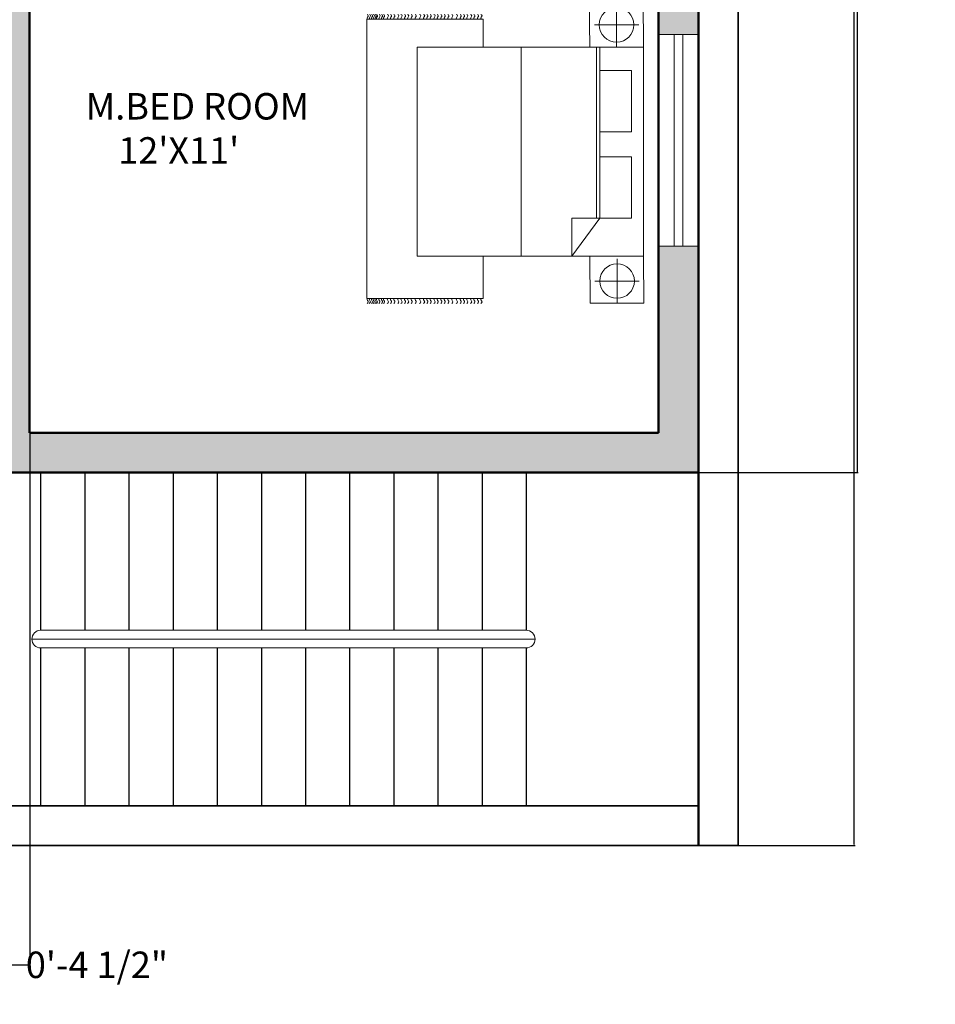
# Model space of a CAD drawing. Units: inches. Extents: x 3398 to 3816, y 15195 to 15771.
# Tile 6 of 10: x 3608 to 3816, y 15195 to 15418. Entities that reach past the tile are written whole.
import ezdxf

# ---------------------------------------------------------------- set-up
doc = ezdxf.new("R2010")
doc.units = ezdxf.units.IN
doc.header["$MEASUREMENT"] = 0
for name, color, linetype, lineweight in [('A-ANNO-DIMS', 2, 'Continuous', 18), ('A-AREA-IDEN', 7, 'Continuous', 25), ('A-FLOR-RAIL', 201, 'Continuous', 18), ('A-FLOR-STRS', 7, 'Continuous', 25), ('A-FURN', 8, 'Continuous', 18), ('A-GLAZ', 4, 'Continuous', 18), ('A-WALL', 7, 'Continuous', 50), ('A-WALL-PATT', 252, 'Continuous', 13), ('C-PROP', 7, 'Continuous', 35)]:
    doc.layers.add(name, color=color, linetype=linetype, lineweight=lineweight)
doc.styles.get("Standard").update_dxf_attribs({"font": 'arial.ttf'})
doc.dimstyles.get("Standard").update_dxf_attribs({"dimtxt": 6, "dimasz": 0.18, "dimexe": 0.18, "dimexo": 0.0625, "dimgap": 0.09, "dimtad": 0, "dimtih": 1, "dimtoh": 1, "dimdec": 1, "dimzin": 0, "dimdsep": 46, "dimlunit": 3, "dimtxsty": 'Standard', "dimcen": 0.09, "dimadec": 0, "dimazin": 0, "dimtfac": 1, "dimtdec": 1, "dimtofl": 0, "dimtmove": 0, "dimatfit": 3, "dimfxl": 1, "dimtolj": 1, "dimtzin": 0, "dimarcsym": 0})

# ---------------------------------------------------------------- blocks, each defined once
blk = doc.blocks.new('*D5')
at = {"layer": 'A-ANNO-DIMS', "color": 0, "lineweight": -2, "transparency": 16777216}
for p, q in [((3771.25, 15739.52), (3797.69, 15739.52)), ((3797.51, 15739.34), (3797.51, 15488.17)), ((3797.51, 15230.7), (3797.51, 15481.87)), ((3771.25, 15230.52), (3797.69, 15230.52))]:
    blk.add_line(p, q, dxfattribs=at)
at = {"layer": 'A-ANNO-DIMS', "color": 0, "transparency": 16777216}
for points in [[(3797.48, 15739.34), (3797.54, 15739.34), (3797.51, 15739.52)], [(3797.48, 15230.7), (3797.54, 15230.7), (3797.51, 15230.52)]]:
    blk.add_solid(points, dxfattribs=at)
at = {"layer": 'Defpoints', "color": 0, "transparency": 16777216}
for p in [(3771.19, 15739.52), (3771.19, 15230.52), (3797.51, 15230.52)]:
    blk.add_point(p, dxfattribs=at)
at = {"layer": 'A-ANNO-DIMS', "color": 0, "transparency": 16777216, "insert": (3797.51, 15485.02), "char_height": 6, "attachment_point": 5}
blk.add_mtext('\\A1;42\'-5.0"', dxfattribs=at)
blk = doc.blocks.new('BED-DOUBLE-WITH-NIGHTSTANDS')
for p, q in [((56.59, 58.08), (56.59, 68.14)), ((0, 64.36), (26.37, 64.36)), ((0, 1.12), (0, 64.36)), ((26.37, 64.36), (26.37, 58.06)), ((61.62, 63.11), (51.56, 63.11)), ((34.96, 10.66), (34.96, 58.08)), ((52, 19.27), (52, 58.08)), ((52.82, 19.32), (52.82, 58.08)), ((52.82, 19.32), (46.47, 10.71)), ((52.82, 19.27), (46.47, 19.27)), ((46.47, 19.27), (46.47, 10.71)), ((26.37, 10.66), (26.37, 1.12)), ((56.69, 0.03), (56.69, 10.09)), ((61.72, 5.06), (51.66, 5.06)), ((26.37, 1.12), (0, 1.12))]:
    blk.add_line(p, q)
for points in [[(50.39, 68.71), (50.5, 58.08), (62.68, 58.08), (62.58, 68.71)], [(62.68, 10.66), (11.37, 10.66), (11.37, 58.08), (62.68, 58.08)], [(59.98, 38.83), (52.82, 38.83), (52.82, 52.73), (59.98, 52.73)], [(59.98, 19.27), (52.82, 19.27), (52.82, 33.16), (59.98, 33.16)], [(50.5, 10.66), (50.6, 0.03), (62.78, 0.03), (62.68, 10.66)]]:
    blk.add_lwpolyline(points, close=True)
for centre in [(56.59, 63.11), (56.69, 5.06)]:
    blk.add_circle(centre, 3.92)
for points, knots in [([(0.07, 65.48), (0.19, 65.39), (0.43, 65.19), (0.19, 64.85), (0.02, 64.57), (0.13, 64.42), (0.18, 64.36)], [0, 0, 0, 0, 0.400747, 0.791423, 1.067667, 1.29709, 1.29709, 1.29709, 1.29709]), ([(0.57, 65.48), (0.7, 65.39), (0.94, 65.19), (0.7, 64.85), (0.52, 64.57), (0.63, 64.42), (0.68, 64.36)], [0, 0, 0, 0, 0.400747, 0.791423, 1.067667, 1.29709, 1.29709, 1.29709, 1.29709]), ([(1.06, 65.48), (1.18, 65.39), (1.42, 65.19), (1.18, 64.85), (1.01, 64.57), (1.11, 64.42), (1.16, 64.36)], [0, 0, 0, 0, 0.400747, 0.791423, 1.067667, 1.29709, 1.29709, 1.29709, 1.29709]), ([(1.46, 65.48), (1.58, 65.39), (1.82, 65.19), (1.58, 64.85), (1.41, 64.57), (1.51, 64.42), (1.56, 64.36)], [0, 0, 0, 0, 0.400747, 0.791423, 1.067667, 1.29709, 1.29709, 1.29709, 1.29709]), ([(1.88, 65.48), (2, 65.39), (2.24, 65.19), (2, 64.85), (1.82, 64.57), (1.93, 64.42), (1.98, 64.36)], [0, 0, 0, 0, 0.400747, 0.791423, 1.067667, 1.29709, 1.29709, 1.29709, 1.29709]), ([(2.18, 65.48), (2.31, 65.39), (2.55, 65.19), (2.31, 64.85), (2.13, 64.57), (2.24, 64.42), (2.29, 64.36)], [0, 0, 0, 0, 0.400747, 0.791423, 1.067667, 1.29709, 1.29709, 1.29709, 1.29709]), ([(2.76, 65.48), (2.88, 65.39), (3.12, 65.19), (2.88, 64.85), (2.71, 64.57), (2.81, 64.42), (2.86, 64.36)], [0, 0, 0, 0, 0.400747, 0.791423, 1.067667, 1.29709, 1.29709, 1.29709, 1.29709]), ([(3.33, 65.48), (3.45, 65.39), (3.7, 65.2), (3.44, 64.85), (3.27, 64.57), (3.38, 64.42), (3.43, 64.36)], [0, 0, 0, 0, 0.407265, 0.802015, 1.07826, 1.307683, 1.307683, 1.307683, 1.307683]), ([(3.75, 65.48), (3.88, 65.39), (4.12, 65.19), (3.88, 64.85), (3.7, 64.57), (3.81, 64.42), (3.86, 64.36)], [0, 0, 0, 0, 0.400747, 0.791423, 1.067667, 1.29709, 1.29709, 1.29709, 1.29709]), ([(4.64, 65.48), (4.76, 65.39), (5, 65.19), (4.76, 64.85), (4.59, 64.57), (4.69, 64.42), (4.74, 64.36)], [0, 0, 0, 0, 0.400747, 0.791423, 1.067667, 1.29709, 1.29709, 1.29709, 1.29709]), ([(5.36, 65.48), (5.49, 65.39), (5.73, 65.19), (5.49, 64.85), (5.31, 64.57), (5.42, 64.42), (5.47, 64.36)], [0, 0, 0, 0, 0.400747, 0.791423, 1.067667, 1.29709, 1.29709, 1.29709, 1.29709]), ([(6.12, 65.48), (6.24, 65.39), (6.48, 65.19), (6.24, 64.85), (6.07, 64.57), (6.17, 64.42), (6.22, 64.36)], [0, 0, 0, 0, 0.400747, 0.791423, 1.067667, 1.29709, 1.29709, 1.29709, 1.29709]), ([(7, 65.48), (7.12, 65.39), (7.36, 65.19), (7.12, 64.85), (6.95, 64.57), (7.05, 64.42), (7.1, 64.36)], [0, 0, 0, 0, 0.400747, 0.791423, 1.067667, 1.29709, 1.29709, 1.29709, 1.29709]), ([(7.73, 65.48), (7.85, 65.39), (8.09, 65.19), (7.85, 64.85), (7.68, 64.57), (7.78, 64.42), (7.83, 64.36)], [0, 0, 0, 0, 0.400747, 0.791423, 1.067667, 1.29709, 1.29709, 1.29709, 1.29709]), ([(8.54, 65.48), (8.66, 65.39), (8.9, 65.19), (8.66, 64.85), (8.49, 64.57), (8.6, 64.42), (8.65, 64.36)], [0, 0, 0, 0, 0.400747, 0.791423, 1.067667, 1.29709, 1.29709, 1.29709, 1.29709]), ([(9.23, 65.48), (9.35, 65.39), (9.59, 65.19), (9.35, 64.85), (9.18, 64.57), (9.29, 64.42), (9.34, 64.36)], [0, 0, 0, 0, 0.400747, 0.791423, 1.067667, 1.29709, 1.29709, 1.29709, 1.29709]), ([(10.05, 65.48), (10.17, 65.39), (10.41, 65.19), (10.17, 64.85), (10, 64.57), (10.1, 64.42), (10.15, 64.36)], [0, 0, 0, 0, 0.400747, 0.791423, 1.067667, 1.29709, 1.29709, 1.29709, 1.29709]), ([(10.93, 65.48), (11.05, 65.39), (11.29, 65.19), (11.05, 64.85), (10.88, 64.57), (10.99, 64.42), (11.03, 64.36)], [0, 0, 0, 0, 0.400747, 0.791423, 1.067667, 1.29709, 1.29709, 1.29709, 1.29709]), ([(11.97, 65.48), (12.09, 65.39), (12.33, 65.19), (12.09, 64.85), (11.92, 64.57), (12.02, 64.42), (12.07, 64.36)], [0, 0, 0, 0, 0.400747, 0.791423, 1.067667, 1.29709, 1.29709, 1.29709, 1.29709]), ([(12.85, 65.48), (12.97, 65.39), (13.21, 65.19), (12.97, 64.85), (12.8, 64.57), (12.9, 64.42), (12.95, 64.36)], [0, 0, 0, 0, 0.400747, 0.791423, 1.067667, 1.29709, 1.29709, 1.29709, 1.29709]), ([(13.58, 65.48), (13.7, 65.39), (13.94, 65.19), (13.7, 64.85), (13.53, 64.57), (13.63, 64.42), (13.68, 64.36)], [0, 0, 0, 0, 0.400747, 0.791423, 1.067667, 1.29709, 1.29709, 1.29709, 1.29709]), ([(14.33, 65.48), (14.45, 65.39), (14.69, 65.19), (14.45, 64.85), (14.28, 64.57), (14.38, 64.42), (14.43, 64.36)], [0, 0, 0, 0, 0.400747, 0.791423, 1.067667, 1.29709, 1.29709, 1.29709, 1.29709]), ([(15.21, 65.48), (15.33, 65.39), (15.57, 65.19), (15.33, 64.85), (15.16, 64.57), (15.27, 64.42), (15.32, 64.36)], [0, 0, 0, 0, 0.400747, 0.791423, 1.067667, 1.29709, 1.29709, 1.29709, 1.29709]), ([(15.94, 65.48), (16.06, 65.39), (16.3, 65.19), (16.06, 64.85), (15.89, 64.57), (16, 64.42), (16.04, 64.36)], [0, 0, 0, 0, 0.400747, 0.791423, 1.067667, 1.29709, 1.29709, 1.29709, 1.29709]), ([(16.76, 65.48), (16.88, 65.39), (17.12, 65.19), (16.88, 64.85), (16.7, 64.57), (16.81, 64.42), (16.86, 64.36)], [0, 0, 0, 0, 0.400747, 0.791423, 1.067667, 1.29709, 1.29709, 1.29709, 1.29709]), ([(17.53, 65.48), (17.65, 65.39), (17.89, 65.19), (17.65, 64.85), (17.48, 64.57), (17.59, 64.42), (17.64, 64.36)], [0, 0, 0, 0, 0.400747, 0.791423, 1.067667, 1.29709, 1.29709, 1.29709, 1.29709]), ([(18.35, 65.48), (18.47, 65.39), (18.71, 65.19), (18.47, 64.85), (18.3, 64.57), (18.4, 64.42), (18.45, 64.36)], [0, 0, 0, 0, 0.400747, 0.791423, 1.067667, 1.29709, 1.29709, 1.29709, 1.29709]), ([(19.23, 65.48), (19.35, 65.39), (19.59, 65.19), (19.35, 64.85), (19.18, 64.57), (19.29, 64.42), (19.33, 64.36)], [0, 0, 0, 0, 0.400747, 0.791423, 1.067667, 1.29709, 1.29709, 1.29709, 1.29709]), ([(20.27, 65.48), (20.39, 65.39), (20.63, 65.19), (20.39, 64.85), (20.22, 64.57), (20.32, 64.42), (20.37, 64.36)], [0, 0, 0, 0, 0.400747, 0.791423, 1.067667, 1.29709, 1.29709, 1.29709, 1.29709]), ([(21.15, 65.48), (21.27, 65.39), (21.51, 65.19), (21.27, 64.85), (21.1, 64.57), (21.21, 64.42), (21.25, 64.36)], [0, 0, 0, 0, 0.400747, 0.791423, 1.067667, 1.29709, 1.29709, 1.29709, 1.29709]), ([(21.88, 65.48), (22, 65.39), (22.24, 65.19), (22, 64.85), (21.83, 64.57), (21.93, 64.42), (21.98, 64.36)], [0, 0, 0, 0, 0.400747, 0.791423, 1.067667, 1.29709, 1.29709, 1.29709, 1.29709]), ([(22.63, 65.48), (22.75, 65.39), (22.99, 65.19), (22.75, 64.85), (22.58, 64.57), (22.69, 64.42), (22.73, 64.36)], [0, 0, 0, 0, 0.400747, 0.791423, 1.067667, 1.29709, 1.29709, 1.29709, 1.29709]), ([(23.51, 65.48), (23.63, 65.39), (23.87, 65.19), (23.63, 64.85), (23.46, 64.57), (23.57, 64.42), (23.62, 64.36)], [0, 0, 0, 0, 0.400747, 0.791423, 1.067667, 1.29709, 1.29709, 1.29709, 1.29709]), ([(24.24, 65.48), (24.36, 65.39), (24.6, 65.19), (24.36, 64.85), (24.19, 64.57), (24.3, 64.42), (24.34, 64.36)], [0, 0, 0, 0, 0.400747, 0.791423, 1.067667, 1.29709, 1.29709, 1.29709, 1.29709]), ([(25.06, 65.48), (25.18, 65.39), (25.42, 65.19), (25.18, 64.85), (25.01, 64.57), (25.11, 64.42), (25.16, 64.36)], [0, 0, 0, 0, 0.400747, 0.791423, 1.067667, 1.29709, 1.29709, 1.29709, 1.29709]), ([(25.84, 65.48), (25.96, 65.39), (26.2, 65.19), (25.96, 64.85), (25.78, 64.57), (25.89, 64.42), (25.94, 64.36)], [0, 0, 0, 0, 0.400747, 0.791423, 1.067667, 1.29709, 1.29709, 1.29709, 1.29709]), ([(0.07, 0), (0.19, 0.1), (0.43, 0.29), (0.19, 0.63), (0.02, 0.91), (0.13, 1.06), (0.18, 1.13)], [0, 0, 0, 0, 0.400747, 0.791423, 1.067667, 1.29709, 1.29709, 1.29709, 1.29709]), ([(0.55, 0), (0.67, 0.1), (0.91, 0.29), (0.67, 0.63), (0.49, 0.91), (0.6, 1.06), (0.65, 1.13)], [0, 0, 0, 0, 0.400747, 0.791423, 1.067667, 1.29709, 1.29709, 1.29709, 1.29709]), ([(1.03, 0), (1.15, 0.1), (1.39, 0.29), (1.15, 0.63), (0.98, 0.91), (1.09, 1.06), (1.13, 1.13)], [0, 0, 0, 0, 0.400747, 0.791423, 1.067667, 1.29709, 1.29709, 1.29709, 1.29709]), ([(1.43, 0), (1.55, 0.1), (1.79, 0.29), (1.55, 0.63), (1.38, 0.91), (1.48, 1.06), (1.53, 1.13)], [0, 0, 0, 0, 0.400747, 0.791423, 1.067667, 1.29709, 1.29709, 1.29709, 1.29709]), ([(1.85, 0), (1.97, 0.1), (2.21, 0.29), (1.97, 0.63), (1.8, 0.91), (1.9, 1.05), (1.94, 1.12)], [0, 0, 0, 0, 0.400747, 0.791423, 1.067667, 1.283686, 1.283686, 1.283686, 1.283686]), ([(2.16, 0), (2.28, 0.1), (2.52, 0.29), (2.28, 0.63), (2.11, 0.91), (2.21, 1.05), (2.25, 1.12)], [0, 0, 0, 0, 0.400747, 0.791423, 1.067667, 1.283686, 1.283686, 1.283686, 1.283686]), ([(2.73, 0), (2.85, 0.1), (3.09, 0.29), (2.85, 0.63), (2.68, 0.91), (2.78, 1.05), (2.82, 1.12)], [0, 0, 0, 0, 0.400747, 0.791423, 1.067667, 1.283686, 1.283686, 1.283686, 1.283686]), ([(3.33, 0), (3.45, 0.1), (3.69, 0.29), (3.45, 0.63), (3.27, 0.91), (3.38, 1.05), (3.42, 1.12)], [0, 0, 0, 0, 0.402903, 0.794912, 1.071156, 1.287177, 1.287177, 1.287177, 1.287177]), ([(3.75, 0), (3.88, 0.1), (4.11, 0.29), (3.88, 0.63), (3.7, 0.91), (3.81, 1.05), (3.85, 1.12)], [0, 0, 0, 0, 0.400747, 0.791423, 1.067667, 1.283686, 1.283686, 1.283686, 1.283686]), ([(4.64, 0), (4.76, 0.1), (5, 0.29), (4.76, 0.63), (4.59, 0.91), (4.69, 1.05), (4.73, 1.12)], [0, 0, 0, 0, 0.400747, 0.791423, 1.067667, 1.283686, 1.283686, 1.283686, 1.283686]), ([(5.36, 0), (5.49, 0.1), (5.73, 0.29), (5.49, 0.63), (5.31, 0.91), (5.42, 1.06), (5.47, 1.13)], [0, 0, 0, 0, 0.400747, 0.791423, 1.067667, 1.29709, 1.29709, 1.29709, 1.29709]), ([(6.12, 0), (6.24, 0.1), (6.48, 0.29), (6.24, 0.63), (6.07, 0.91), (6.17, 1.06), (6.22, 1.13)], [0, 0, 0, 0, 0.400747, 0.791423, 1.067667, 1.29709, 1.29709, 1.29709, 1.29709]), ([(7, 0), (7.12, 0.1), (7.36, 0.29), (7.12, 0.63), (6.95, 0.91), (7.05, 1.06), (7.1, 1.13)], [0, 0, 0, 0, 0.400747, 0.791423, 1.067667, 1.29709, 1.29709, 1.29709, 1.29709]), ([(7.73, 0), (7.85, 0.1), (8.09, 0.29), (7.85, 0.63), (7.68, 0.91), (7.78, 1.06), (7.83, 1.13)], [0, 0, 0, 0, 0.400747, 0.791423, 1.067667, 1.29709, 1.29709, 1.29709, 1.29709]), ([(8.54, 0), (8.66, 0.1), (8.9, 0.29), (8.66, 0.63), (8.49, 0.91), (8.6, 1.06), (8.65, 1.13)], [0, 0, 0, 0, 0.400747, 0.791423, 1.067667, 1.29709, 1.29709, 1.29709, 1.29709]), ([(9.23, 0), (9.35, 0.1), (9.59, 0.29), (9.35, 0.63), (9.18, 0.91), (9.29, 1.06), (9.34, 1.13)], [0, 0, 0, 0, 0.400747, 0.791423, 1.067667, 1.29709, 1.29709, 1.29709, 1.29709]), ([(10.05, 0), (10.17, 0.1), (10.41, 0.29), (10.17, 0.63), (10, 0.91), (10.1, 1.06), (10.15, 1.13)], [0, 0, 0, 0, 0.400747, 0.791423, 1.067667, 1.29709, 1.29709, 1.29709, 1.29709]), ([(10.93, 0), (11.05, 0.1), (11.29, 0.29), (11.05, 0.63), (10.88, 0.91), (10.99, 1.06), (11.03, 1.13)], [0, 0, 0, 0, 0.400747, 0.791423, 1.067667, 1.29709, 1.29709, 1.29709, 1.29709]), ([(11.97, 0), (12.09, 0.1), (12.33, 0.29), (12.09, 0.63), (11.92, 0.91), (12.02, 1.06), (12.07, 1.13)], [0, 0, 0, 0, 0.400747, 0.791423, 1.067667, 1.29709, 1.29709, 1.29709, 1.29709]), ([(12.85, 0), (12.97, 0.1), (13.21, 0.29), (12.97, 0.63), (12.8, 0.91), (12.9, 1.06), (12.95, 1.13)], [0, 0, 0, 0, 0.400747, 0.791423, 1.067667, 1.29709, 1.29709, 1.29709, 1.29709]), ([(13.58, 0), (13.7, 0.1), (13.94, 0.29), (13.7, 0.63), (13.53, 0.91), (13.63, 1.06), (13.68, 1.13)], [0, 0, 0, 0, 0.400747, 0.791423, 1.067667, 1.29709, 1.29709, 1.29709, 1.29709]), ([(14.33, 0), (14.45, 0.1), (14.69, 0.29), (14.45, 0.63), (14.28, 0.91), (14.38, 1.06), (14.43, 1.13)], [0, 0, 0, 0, 0.400747, 0.791423, 1.067667, 1.29709, 1.29709, 1.29709, 1.29709]), ([(15.21, 0), (15.33, 0.1), (15.57, 0.29), (15.33, 0.63), (15.16, 0.91), (15.27, 1.06), (15.32, 1.13)], [0, 0, 0, 0, 0.400747, 0.791423, 1.067667, 1.29709, 1.29709, 1.29709, 1.29709]), ([(15.94, 0), (16.06, 0.1), (16.3, 0.29), (16.06, 0.63), (15.89, 0.91), (16, 1.06), (16.04, 1.13)], [0, 0, 0, 0, 0.400747, 0.791423, 1.067667, 1.29709, 1.29709, 1.29709, 1.29709]), ([(16.76, 0), (16.88, 0.1), (17.12, 0.29), (16.88, 0.63), (16.7, 0.91), (16.81, 1.06), (16.86, 1.13)], [0, 0, 0, 0, 0.400747, 0.791423, 1.067667, 1.29709, 1.29709, 1.29709, 1.29709]), ([(17.53, 0), (17.65, 0.1), (17.89, 0.29), (17.65, 0.63), (17.48, 0.91), (17.59, 1.06), (17.64, 1.13)], [0, 0, 0, 0, 0.400747, 0.791423, 1.067667, 1.29709, 1.29709, 1.29709, 1.29709]), ([(18.35, 0), (18.47, 0.1), (18.71, 0.29), (18.47, 0.63), (18.3, 0.91), (18.4, 1.06), (18.45, 1.13)], [0, 0, 0, 0, 0.400747, 0.791423, 1.067667, 1.29709, 1.29709, 1.29709, 1.29709]), ([(19.23, 0), (19.35, 0.1), (19.59, 0.29), (19.35, 0.63), (19.18, 0.91), (19.29, 1.06), (19.33, 1.13)], [0, 0, 0, 0, 0.400747, 0.791423, 1.067667, 1.29709, 1.29709, 1.29709, 1.29709]), ([(20.27, 0), (20.39, 0.1), (20.63, 0.29), (20.39, 0.63), (20.22, 0.91), (20.32, 1.06), (20.37, 1.13)], [0, 0, 0, 0, 0.400747, 0.791423, 1.067667, 1.29709, 1.29709, 1.29709, 1.29709]), ([(21.15, 0), (21.27, 0.1), (21.51, 0.29), (21.27, 0.63), (21.1, 0.91), (21.21, 1.06), (21.25, 1.13)], [0, 0, 0, 0, 0.400747, 0.791423, 1.067667, 1.29709, 1.29709, 1.29709, 1.29709]), ([(21.88, 0), (22, 0.1), (22.24, 0.29), (22, 0.63), (21.83, 0.91), (21.93, 1.06), (21.98, 1.13)], [0, 0, 0, 0, 0.400747, 0.791423, 1.067667, 1.29709, 1.29709, 1.29709, 1.29709]), ([(22.63, 0), (22.75, 0.1), (22.99, 0.29), (22.75, 0.63), (22.58, 0.91), (22.69, 1.06), (22.73, 1.13)], [0, 0, 0, 0, 0.400747, 0.791423, 1.067667, 1.29709, 1.29709, 1.29709, 1.29709]), ([(23.51, 0), (23.63, 0.1), (23.87, 0.29), (23.63, 0.63), (23.46, 0.91), (23.57, 1.06), (23.62, 1.13)], [0, 0, 0, 0, 0.400747, 0.791423, 1.067667, 1.29709, 1.29709, 1.29709, 1.29709]), ([(24.24, 0), (24.36, 0.1), (24.6, 0.29), (24.36, 0.63), (24.19, 0.91), (24.3, 1.06), (24.34, 1.13)], [0, 0, 0, 0, 0.400747, 0.791423, 1.067667, 1.29709, 1.29709, 1.29709, 1.29709]), ([(25.06, 0), (25.18, 0.1), (25.42, 0.29), (25.18, 0.63), (25.01, 0.91), (25.11, 1.06), (25.16, 1.13)], [0, 0, 0, 0, 0.400747, 0.791423, 1.067667, 1.29709, 1.29709, 1.29709, 1.29709]), ([(25.84, 0), (25.96, 0.1), (26.2, 0.29), (25.96, 0.63), (25.78, 0.91), (25.89, 1.06), (25.94, 1.13)], [0, 0, 0, 0, 0.400747, 0.791423, 1.067667, 1.29709, 1.29709, 1.29709, 1.29709])]:
    blk.add_open_spline(points, degree=3, knots=knots)
blk = doc.blocks.new('*D37')
at = {"layer": 'A-ANNO-DIMS', "color": 0, "lineweight": -2, "transparency": 16777216}
for p, q in [((3762.25, 15730.52), (3798.42, 15730.52)), ((3798.24, 15730.34), (3798.24, 15525.96)), ((3798.24, 15315.2), (3798.24, 15519.58)), ((3762.25, 15315.02), (3798.42, 15315.02))]:
    blk.add_line(p, q, dxfattribs=at)
at = {"layer": 'A-ANNO-DIMS', "color": 0, "transparency": 16777216}
for points in [[(3798.21, 15730.34), (3798.27, 15730.34), (3798.24, 15730.52)], [(3798.21, 15315.2), (3798.27, 15315.2), (3798.24, 15315.02)]]:
    blk.add_solid(points, dxfattribs=at)
at = {"layer": 'Defpoints', "color": 0, "transparency": 16777216}
for p in [(3762.19, 15730.52), (3798.24, 15730.52), (3762.19, 15315.02)]:
    blk.add_point(p, dxfattribs=at)
at = {"layer": 'A-ANNO-DIMS', "color": 0, "transparency": 16777216, "insert": (3798.24, 15522.77), "char_height": 6, "attachment_point": 5}
blk.add_mtext('\\A1;34\'-7 1/2"', dxfattribs=at)
blk = doc.blocks.new('*D42')
at = {"layer": 'A-ANNO-DIMS', "color": 0, "lineweight": -2, "transparency": 16777216}
for p, q in [((3606.19, 15698.39), (3606.19, 15203.29)), ((3610.7, 15698.39), (3610.7, 15203.29)), ((3606.37, 15203.47), (3610.52, 15203.47)), ((3610.7, 15203.47), (3610.88, 15203.47))]:
    blk.add_line(p, q, dxfattribs=at)
at = {"layer": 'A-ANNO-DIMS', "color": 0, "transparency": 16777216}
for points in [[(3606.37, 15203.5), (3606.37, 15203.44), (3606.19, 15203.47)], [(3610.52, 15203.5), (3610.52, 15203.44), (3610.7, 15203.47)]]:
    blk.add_solid(points, dxfattribs=at)
at = {"layer": 'Defpoints', "color": 0, "transparency": 16777216}
for p in [(3606.19, 15698.45), (3610.7, 15698.45), (3610.7, 15203.47)]:
    blk.add_point(p, dxfattribs=at)
at = {"layer": 'A-ANNO-DIMS', "color": 0, "transparency": 16777216, "insert": (3625.93, 15203.47), "char_height": 6, "attachment_point": 5}
blk.add_mtext('\\A1;0\'-4 1/2"', dxfattribs=at)

msp = doc.modelspace()

# ---------------------------------------------------------------- hatches: boundary and pattern name
at = {"layer": 'A-WALL-PATT'}
h = msp.add_hatch(color=256, dxfattribs=at)
h.dxf.hatch_style = 1
h.paths.add_polyline_path([(3515.96, 15730.52), (3465.19, 15730.52), (3465.19, 15715.52), (3474.19, 15715.52), (3474.19, 15721.52), (3515.96, 15721.52)])
h.paths.add_polyline_path([(3719.81, 15730.52), (3675.76, 15730.52), (3675.76, 15721.52), (3700.69, 15721.52), (3700.69, 15637.52), (3610.69, 15637.52), (3610.69, 15663.97), (3606.19, 15663.97), (3606.19, 15601.52), (3599.08, 15601.52), (3599.08, 15592.52), (3606.19, 15592.52), (3606.19, 15508.52), (3616.69, 15508.52), (3616.69, 15513.02), (3610.69, 15513.02), (3610.69, 15633.02), (3708.19, 15633.02), (3708.19, 15637.52), (3705.19, 15637.52), (3705.19, 15721.52), (3719.81, 15721.52)])
h.paths.add_polyline_path([(3762.19, 15730.52), (3743.77, 15730.52), (3743.77, 15721.52), (3753.19, 15721.52), (3753.19, 15637.52), (3732.19, 15637.52), (3732.19, 15633.02), (3753.19, 15633.02), (3753.19, 15597.39), (3762.19, 15597.39)])
h.paths.add_polyline_path([(3762.19, 15549.39), (3753.19, 15549.39), (3753.19, 15513.02), (3652.69, 15513.02), (3652.69, 15508.52), (3664.69, 15508.52), (3664.69, 15460.52), (3652.69, 15460.52), (3652.69, 15456.02), (3672.19, 15456.02), (3672.19, 15460.52), (3669.19, 15460.52), (3669.19, 15508.52), (3753.19, 15508.52), (3753.19, 15497.51), (3762.19, 15497.51)])
h.paths.add_polyline_path([(3762.19, 15473.48), (3753.19, 15473.48), (3753.19, 15460.52), (3696.19, 15460.52), (3696.19, 15456.02), (3753.19, 15456.02), (3753.19, 15414.25), (3762.19, 15414.25)])
h.paths.add_polyline_path([(3762.19, 15366.28), (3753.19, 15366.28), (3753.19, 15324.02), (3610.69, 15324.02), (3610.69, 15456.02), (3616.69, 15456.02), (3616.69, 15460.52), (3610.69, 15460.52), (3606.19, 15460.52), (3606.19, 15382.52), (3587.73, 15382.52), (3587.73, 15373.52), (3606.19, 15373.52), (3606.19, 15315.02), (3762.19, 15315.02)])
h.paths.add_polyline_path([(3539.73, 15382.52), (3522.19, 15382.52), (3522.19, 15373.52), (3539.73, 15373.52)])
h.paths.add_polyline_path([(3480.19, 15382.52), (3474.19, 15382.52), (3474.19, 15452.47), (3465.19, 15452.47), (3465.19, 15373.52), (3480.19, 15373.52)])
h.paths.add_polyline_path([(3551.04, 15601.52), (3474.19, 15601.52), (3474.19, 15679.52), (3465.19, 15679.52), (3465.19, 15500.47), (3474.19, 15500.47), (3474.19, 15592.52), (3551.04, 15592.52)])

# ---------------------------------------------------------------- linework, layer by layer
at = {"layer": 'A-FLOR-RAIL'}
for p, q in [((3723.19, 15279.27), (3613.19, 15279.27)), ((3725.19, 15277.27), (3611.19, 15277.27)), ((3723.19, 15277.27), (3613.19, 15277.27)), ((3723.19, 15275.27), (3613.19, 15275.27))]:
    msp.add_line(p, q, dxfattribs=at)
for centre, start, end in [((3613.19, 15277.27), 90, 270), ((3723.19, 15277.27), 270, 90)]:
    msp.add_arc(centre, 2, start, end, dxfattribs=at)
at = {"layer": 'A-FLOR-STRS'}
for p, q in [((3613.19, 15315.02), (3613.19, 15279.27)), ((3623.19, 15315.02), (3623.19, 15279.27)), ((3633.19, 15315.02), (3633.19, 15279.27)), ((3643.19, 15315.02), (3643.19, 15279.27)), ((3653.19, 15315.02), (3653.19, 15279.27)), ((3663.19, 15315.02), (3663.19, 15279.27)), ((3673.19, 15315.02), (3673.19, 15279.27)), ((3683.19, 15315.02), (3683.19, 15279.27)), ((3693.19, 15315.02), (3693.19, 15279.27)), ((3703.19, 15315.02), (3703.19, 15279.27)), ((3713.19, 15315.02), (3713.19, 15279.27)), ((3726.19, 15315.02), (3723.19, 15315.02)), ((3723.19, 15315.02), (3723.19, 15279.27)), ((3762.19, 15315.02), (3726.19, 15315.02)), ((3613.19, 15275.27), (3613.19, 15239.52)), ((3623.19, 15275.27), (3623.19, 15239.52)), ((3633.19, 15275.27), (3633.19, 15239.52)), ((3643.19, 15275.27), (3643.19, 15239.52)), ((3653.19, 15275.27), (3653.19, 15239.52)), ((3663.19, 15275.27), (3663.19, 15239.52)), ((3673.19, 15275.27), (3673.19, 15239.52)), ((3683.19, 15275.27), (3683.19, 15239.52)), ((3693.19, 15275.27), (3693.19, 15239.52)), ((3703.19, 15275.27), (3703.19, 15239.52)), ((3713.19, 15275.27), (3713.19, 15239.52)), ((3723.19, 15275.27), (3723.19, 15239.52))]:
    msp.add_line(p, q, dxfattribs=at)
at = {"layer": 'A-GLAZ'}
for p, q in [((3753.19, 15414.25), (3762.19, 15414.25)), ((3753.19, 15366.28), (3753.19, 15414.25)), ((3756.69, 15366.28), (3756.69, 15414.25)), ((3758.69, 15414.25), (3758.69, 15366.28)), ((3762.19, 15414.25), (3762.19, 15366.28)), ((3762.19, 15366.28), (3753.19, 15366.28))]:
    msp.add_line(p, q, dxfattribs=at)
at = {"layer": 'A-WALL'}
for p, q in [((3762.19, 15730.52), (3762.19, 15230.52)), ((3610.69, 15456.02), (3610.69, 15324.02)), ((3753.19, 15456.02), (3753.19, 15324.02)), ((3610.69, 15324.02), (3753.19, 15324.02)), ((3606.19, 15315.02), (3762.19, 15315.02))]:
    msp.add_line(p, q, dxfattribs=at)
at = {"layer": 'C-PROP'}
for p, q in [((3771.19, 15739.52), (3771.19, 15230.52)), ((3452.19, 15239.52), (3762.19, 15239.52)), ((3443.19, 15230.52), (3771.19, 15230.52))]:
    msp.add_line(p, q, dxfattribs=at)

# ---------------------------------------------------------------- block references
at = {"layer": 'A-FURN'}
msp.add_blockref('BED-DOUBLE-WITH-NIGHTSTANDS', (3687.08, 15353.35), dxfattribs=at)

# ---------------------------------------------------------------- texts
at = {"layer": 'A-AREA-IDEN', "insert": (3623.42, 15401), "char_height": 6, "attachment_point": 1}
msp.add_mtext_dynamic_manual_height_columns("M.BED ROOM\\P    12'X11'", width=81.4286, gutter_width=30, heights=[0], dxfattribs=at)

# ---------------------------------------------------------------- dimensions: what is measured, and where the dimension line sits
at = {"layer": 'A-ANNO-DIMS'}
for base, p1, p2, override, picture, middle in [((3797.51, 15230.52), (3771.19, 15739.52), (3771.19, 15230.52), {"dimclrd": 0, "dimclre": 0, "dimclrt": 0}, '*D5', (3797.51, 15485.02)), ((3798.24, 15730.52), (3762.19, 15315.02), (3762.19, 15730.52), {"dimdec": 1, "dimlfac": 1, "dimrnd": 0, "dimzin": 1, "dimdsep": 46, "dimlunit": 4, "dimfrac": 2}, '*D37', (3798.24, 15522.77))]:
    dim = msp.add_linear_dim(base=base, p1=p1, p2=p2, angle=90, dimstyle='Standard', override=override, dxfattribs=at)
    dim.commit()
    dim.dimension.update_dxf_attribs({"geometry": picture, "text_midpoint": middle})
dim = msp.add_linear_dim(base=(3610.7, 15203.47), p1=(3606.19, 15698.45), p2=(3610.7, 15698.45), dimstyle='Standard', override={"dimdec": 1, "dimlfac": 1, "dimrnd": 0, "dimzin": 1, "dimdsep": 46, "dimlunit": 4, "dimfrac": 2}, dxfattribs=at)
dim.commit()
dim.dimension.update_dxf_attribs({"geometry": '*D42', "text_midpoint": (3625.93, 15203.47)})

doc.saveas('drawing.dxf')
